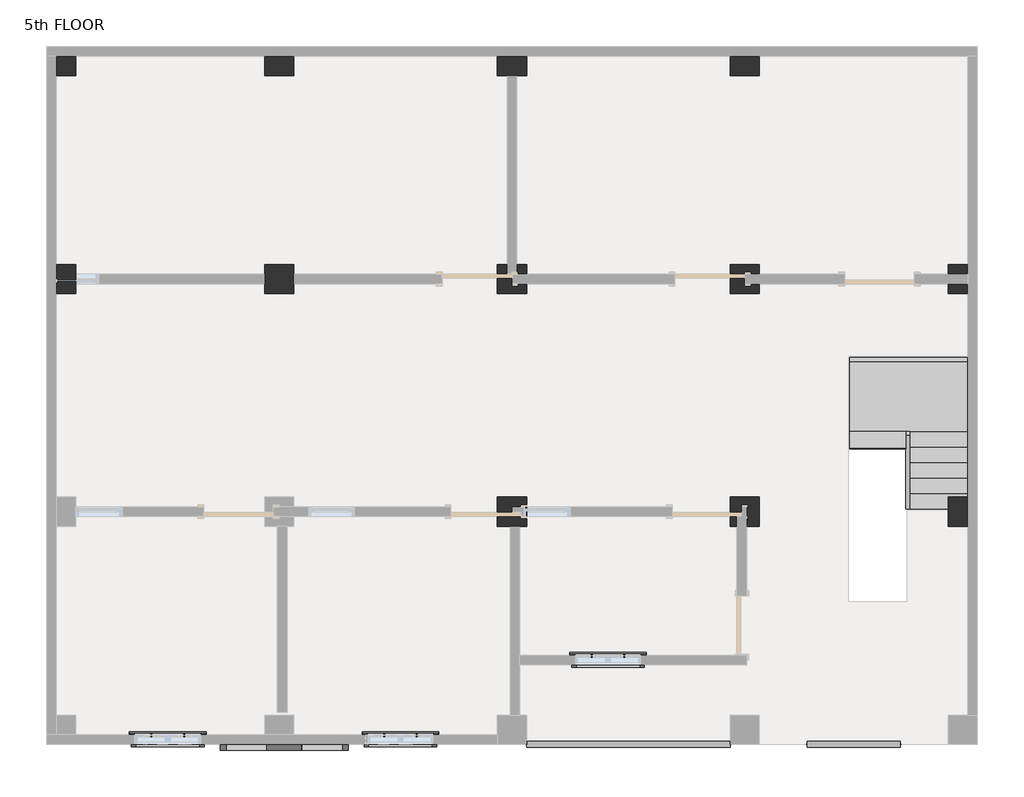
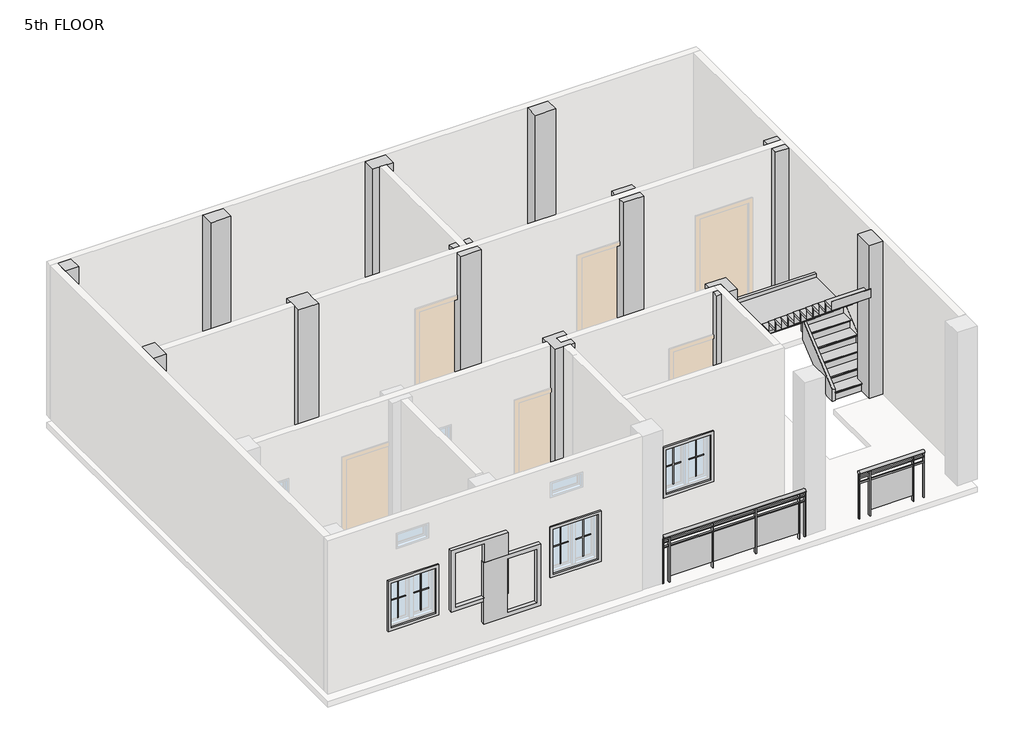
# One storey, part 2 of 2: 12 columns, 12 proxies, 4 members, 2 railings, 1 damper, 1 stair flight.
"""IFC4 building model written with IfcOpenShell, lengths in millimetres."""

from ifc_helpers import new_model, si_unit, point, frame, origin, place, context, project, spatial, polyline, ellipse_curve, trimmed, outline, extrude, faceted_brep, transform, mapped, element, save
from ifc_brep_helpers import plane_surface, extruded_surface, advanced_brep
from components import muntin_pattern_2x2_muntin_pattern_2x2_b3fe6957, muntin_pattern_2x2_muntin_pattern_2x2_3e0ecaf2, trim_window_exterior_flat_with_sill_41619996, trim_window_interior_flat_picture_frame_51c85655, duct_accessories_8_duct_accessories_1_4ac22e68, stair_flight_9ad1fb7f

model = new_model("IFC4")

# Units and contexts
model_context = context("Model", 3, world=origin())
ifc_project = project(units=[si_unit("LENGTHUNIT", "METRE", prefix="MILLI")], contexts=[model_context])

# Site, building, storey
site = spatial("IfcSite", under=ifc_project)
building = spatial("IfcBuilding", under=site)
storey = spatial("IfcBuildingStorey", under=building, Name="5th FLOOR", Elevation=15087.6)

# Proxies
placement = place(None, origin())
muntin_pattern_2x2_muntin_pattern_2x2_shape = muntin_pattern_2x2_muntin_pattern_2x2_b3fe6957(model_context)
element("IfcBuildingElementProxy", 1, Name="Muntin Pattern_2x2 : Muntin Pattern_2x2", ObjectType="Muntin Pattern_2x2 : Muntin Pattern_2x2", at=placement, inside=storey, context=model_context, shape_type="MappedRepresentation", body=[
    mapped(muntin_pattern_2x2_muntin_pattern_2x2_shape, transform((-14441.409625, -253.8184478, 16071.85), x_axis=(1.0, 0.0, 0.0), y_axis=(0.0, 1.0, 0.0), z_axis=(0.0, 0.0, 1.0))),
])
element("IfcBuildingElementProxy", 2, Name="Muntin Pattern_2x2 : Muntin Pattern_2x2", ObjectType="Muntin Pattern_2x2 : Muntin Pattern_2x2", at=placement, inside=storey, context=model_context, shape_type="MappedRepresentation", body=[
    mapped(muntin_pattern_2x2_muntin_pattern_2x2_shape, transform((-11393.409625, -253.8184478, 16071.85), x_axis=(1.0, 0.0, 0.0), y_axis=(0.0, 1.0, 0.0), z_axis=(0.0, 0.0, 1.0))),
])
element("IfcBuildingElementProxy", 3, Name="Muntin Pattern_2x2 : Muntin Pattern_2x2", ObjectType="Muntin Pattern_2x2 : Muntin Pattern_2x2", at=placement, inside=storey, context=model_context, shape_type="MappedRepresentation", body=[
    mapped(muntin_pattern_2x2_muntin_pattern_2x2_shape, transform((-8675.609625, 787.5815522, 16071.85), x_axis=(1.0, 0.0, 0.0), y_axis=(0.0, 1.0, 0.0), z_axis=(0.0, 0.0, 1.0))),
])
muntin_pattern_2x2_muntin_pattern_2x2_2_shape = muntin_pattern_2x2_muntin_pattern_2x2_3e0ecaf2(model_context)
element("IfcBuildingElementProxy", 4, Name="Muntin Pattern_2x2 : Muntin Pattern_2x2", ObjectType="Muntin Pattern_2x2 : Muntin Pattern_2x2", at=placement, inside=storey, context=model_context, shape_type="MappedRepresentation", body=[
    mapped(muntin_pattern_2x2_muntin_pattern_2x2_2_shape, transform((-14012.784625, -253.8184478, 16071.85), x_axis=(-1.0, 0.0, 0.0), y_axis=(0.0, -1.0, 0.0), z_axis=(0.0, 0.0, 1.0))),
])
element("IfcBuildingElementProxy", 5, Name="Muntin Pattern_2x2 : Muntin Pattern_2x2", ObjectType="Muntin Pattern_2x2 : Muntin Pattern_2x2", at=placement, inside=storey, context=model_context, shape_type="MappedRepresentation", body=[
    mapped(muntin_pattern_2x2_muntin_pattern_2x2_2_shape, transform((-10964.784625, -253.8184478, 16071.85), x_axis=(-1.0, 0.0, 0.0), y_axis=(0.0, -1.0, 0.0), z_axis=(0.0, 0.0, 1.0))),
])
element("IfcBuildingElementProxy", 6, Name="Muntin Pattern_2x2 : Muntin Pattern_2x2", ObjectType="Muntin Pattern_2x2 : Muntin Pattern_2x2", at=placement, inside=storey, context=model_context, shape_type="MappedRepresentation", body=[
    mapped(muntin_pattern_2x2_muntin_pattern_2x2_2_shape, transform((-8246.984625, 787.5815522, 16071.85), x_axis=(-1.0, 0.0, 0.0), y_axis=(0.0, -1.0, 0.0), z_axis=(0.0, 0.0, 1.0))),
])
trim_window_exterior_flat_with_sill_shape = trim_window_exterior_flat_with_sill_41619996(model_context)
element("IfcBuildingElementProxy", 7, Name="Trim-Window-Exterior-Flat : with Sill", ObjectType="Trim-Window-Exterior-Flat : with Sill", at=placement, inside=storey, context=model_context, shape_type="MappedRepresentation", body=[
    mapped(trim_window_exterior_flat_with_sill_shape, transform((-14227.097125, -244.2934478, 16916.4), x_axis=(-1.0, 0.0, 0.0), y_axis=(0.0, 0.0, 1.0), z_axis=(0.0, 1.0, 0.0))),
])
element("IfcBuildingElementProxy", 8, Name="Trim-Window-Exterior-Flat : with Sill", ObjectType="Trim-Window-Exterior-Flat : with Sill", at=placement, inside=storey, context=model_context, shape_type="MappedRepresentation", body=[
    mapped(trim_window_exterior_flat_with_sill_shape, transform((-11179.097125, -244.2934478, 16916.4), x_axis=(-1.0, 0.0, 0.0), y_axis=(0.0, 0.0, 1.0), z_axis=(0.0, 1.0, 0.0))),
])
element("IfcBuildingElementProxy", 9, Name="Trim-Window-Exterior-Flat : with Sill", ObjectType="Trim-Window-Exterior-Flat : with Sill", at=placement, inside=storey, context=model_context, shape_type="MappedRepresentation", body=[
    mapped(trim_window_exterior_flat_with_sill_shape, transform((-8461.297125, 797.1065522, 16916.4), x_axis=(-1.0, 0.0, 0.0), y_axis=(0.0, 0.0, 1.0), z_axis=(0.0, 1.0, 0.0))),
])
trim_window_interior_flat_picture_frame_shape = trim_window_interior_flat_picture_frame_51c85655(model_context)
element("IfcBuildingElementProxy", 10, Name="Trim-Window-Interior-Flat : Picture Frame", ObjectType="Trim-Window-Interior-Flat : Picture Frame", at=placement, inside=storey, context=model_context, shape_type="MappedRepresentation", body=[
    mapped(trim_window_interior_flat_picture_frame_shape, transform((-14227.097125, -371.2934478, 16916.4), x_axis=(1.0, 0.0, 0.0), y_axis=(0.0, 0.0, 1.0), z_axis=(0.0, -1.0, 0.0))),
])
element("IfcBuildingElementProxy", 11, Name="Trim-Window-Interior-Flat : Picture Frame", ObjectType="Trim-Window-Interior-Flat : Picture Frame", at=placement, inside=storey, context=model_context, shape_type="MappedRepresentation", body=[
    mapped(trim_window_interior_flat_picture_frame_shape, transform((-11179.097125, -371.2934478, 16916.4), x_axis=(1.0, 0.0, 0.0), y_axis=(0.0, 0.0, 1.0), z_axis=(0.0, -1.0, 0.0))),
])
element("IfcBuildingElementProxy", 12, Name="Trim-Window-Interior-Flat : Picture Frame", ObjectType="Trim-Window-Interior-Flat : Picture Frame", at=placement, inside=storey, context=model_context, shape_type="MappedRepresentation", body=[
    mapped(trim_window_interior_flat_picture_frame_shape, transform((-8461.297125, 670.1065522, 16916.4), x_axis=(1.0, 0.0, 0.0), y_axis=(0.0, 0.0, 1.0), z_axis=(0.0, -1.0, 0.0))),
])

# Columns
element("IfcColumn", 13, ObjectType="column family : column family", at=placement, inside=storey, context=model_context, shape_type="SweptSolid", body=[
    extrude(outline(polyline([(-15433.597125, 8645.7065522), (-15433.597125, 8391.7065522), (-15687.597125, 8391.7065522), (-15687.597125, 8645.7065522), (-15433.597125, 8645.7065522)])), frame((0.0, 0.0, 15092.6), z_axis=(0.0, 0.0, 1.0), x_axis=(1.0, 0.0, 0.0)), (0.0, 0.0, 1.0), 3038.0),
])
element("IfcColumn", 14, ObjectType="column family : column family", at=placement, inside=storey, context=model_context, shape_type="SweptSolid", body=[
    extrude(outline(polyline([(-12576.097125, 5915.2065522), (-12576.097125, 5534.2065522), (-12957.097125, 5534.2065522), (-12957.097125, 5915.2065522), (-12576.097125, 5915.2065522)])), frame((0.0, 0.0, 15092.6), z_axis=(0.0, 0.0, 1.0), x_axis=(1.0, 0.0, 0.0)), (0.0, 0.0, 1.0), 3038.0),
])
element("IfcColumn", 15, ObjectType="column family : column family", at=placement, inside=storey, context=model_context, shape_type="Brep", body=[
    faceted_brep([(-9655.097125, 5915.2065522, 15092.6), (-9528.097125, 5915.2065522, 15092.6), (-9528.097125, 5788.2065522, 15092.6), (-9655.097125, 5788.2065522, 15092.6), (-9528.097125, 5915.2065522, 18130.6), (-9655.097125, 5915.2065522, 18130.6), (-9655.097125, 5788.2065522, 18130.6), (-9528.097125, 5788.2065522, 18130.6)], [[[0, 1, 2, 3]], [[4, 5, 6, 7]], [[0, 3, 6, 5]], [[4, 1, 0, 5]], [[3, 2, 7, 6]], [[1, 4, 7, 2]]]),
    faceted_brep([(-9528.097125, 5534.2065522, 18130.6), (-9528.097125, 5534.2065522, 15092.6), (-9528.097125, 5661.2065522, 15092.6), (-9528.097125, 5661.2065522, 18130.6), (-9909.097125, 5534.2065522, 15092.6), (-9909.097125, 5534.2065522, 18130.6), (-9909.097125, 5915.2065522, 15092.6), (-9909.097125, 5661.2065522, 18130.6), (-9909.097125, 5661.2065522, 17221.2), (-9909.097125, 5788.2065522, 17221.2), (-9909.097125, 5788.2065522, 18130.6), (-9909.097125, 5915.2065522, 18130.6), (-9782.097125, 5915.2065522, 18130.6), (-9782.097125, 5915.2065522, 15092.6), (-9782.097125, 5788.2065522, 15092.6), (-9782.097125, 5788.2065522, 18130.6), (-9782.097125, 5788.2065522, 17221.2), (-9718.597125, 5788.2065522, 15092.6), (-9718.597125, 5788.2065522, 17221.2), (-9718.597125, 5661.2065522, 15092.6), (-9718.597125, 5661.2065522, 17221.2)], [[[0, 1, 2, 3]], [[4, 1, 0, 5]], [[6, 4, 5, 7, 8, 9, 10, 11]], [[6, 11, 12, 13]], [[14, 13, 12, 15, 16]], [[17, 14, 16, 18]], [[19, 20, 8, 7, 3, 2]], [[1, 4, 6, 13, 14, 17, 19, 2]], [[5, 0, 3, 7]], [[12, 11, 10, 15]], [[9, 16, 15, 10]], [[18, 20, 19, 17]], [[20, 18, 16, 9, 8]]]),
])
element("IfcColumn", 16, ObjectType="column family : column family", at=placement, inside=storey, context=model_context, shape_type="Brep", body=[
    faceted_brep([(-6480.097125, 5534.2065522, 15092.6), (-6861.097125, 5534.2065522, 15092.6), (-6861.097125, 5915.2065522, 15092.6), (-6480.097125, 5915.2065522, 15092.6), (-6480.097125, 5788.2065522, 15092.6), (-6670.597125, 5788.2065522, 15092.6), (-6670.597125, 5661.2065522, 15092.6), (-6480.097125, 5661.2065522, 15092.6), (-6480.097125, 5534.2065522, 18130.6), (-6480.097125, 5661.2065522, 18130.6), (-6861.097125, 5534.2065522, 18130.6), (-6861.097125, 5661.2065522, 18130.6), (-6861.097125, 5661.2065522, 17221.2), (-6861.097125, 5788.2065522, 17221.2), (-6861.097125, 5788.2065522, 18130.6), (-6861.097125, 5915.2065522, 18130.6), (-6480.097125, 5915.2065522, 18130.6), (-6670.597125, 5661.2065522, 17221.2), (-6670.597125, 5788.2065522, 17221.2), (-6480.097125, 5788.2065522, 18130.6)], [[[0, 1, 2, 3, 4, 5, 6, 7]], [[8, 0, 7, 9]], [[1, 0, 8, 10]], [[2, 1, 10, 11, 12, 13, 14, 15]], [[3, 2, 15, 16]], [[10, 8, 9, 11]], [[6, 17, 12, 11, 9, 7]], [[13, 18, 5, 4, 19, 14]], [[3, 16, 19, 4]], [[16, 15, 14, 19]], [[18, 17, 6, 5]], [[17, 18, 13, 12]]]),
])
element("IfcColumn", 17, ObjectType="column family : column family", at=placement, inside=storey, context=model_context, shape_type="Brep", body=[
    faceted_brep([(-6480.097125, 2867.2065522, 15092.6), (-6480.097125, 2486.2065522, 15092.6), (-6645.197125, 2486.2065522, 15092.6), (-6645.197125, 2740.2065522, 15092.6), (-6708.697125, 2740.2065522, 15092.6), (-6708.697125, 2613.2065522, 15092.6), (-6772.197125, 2613.2065522, 15092.6), (-6772.197125, 2486.2065522, 15092.6), (-6861.097125, 2486.2065522, 15092.6), (-6861.097125, 2867.2065522, 15092.6), (-6480.097125, 2867.2065522, 18130.6), (-6480.097125, 2486.2065522, 18130.6), (-6861.097125, 2486.2065522, 18130.6), (-6772.197125, 2486.2065522, 18130.6), (-6861.097125, 2613.2065522, 18130.6), (-6861.097125, 2613.2065522, 17221.2), (-6861.097125, 2740.2065522, 17221.2), (-6861.097125, 2740.2065522, 18130.6), (-6861.097125, 2867.2065522, 18130.6), (-6772.197125, 2740.2065522, 18130.6), (-6645.197125, 2740.2065522, 18130.6), (-6645.197125, 2486.2065522, 18130.6), (-6772.197125, 2613.2065522, 18130.6), (-6772.197125, 2613.2065522, 17221.2), (-6772.197125, 2740.2065522, 17221.2), (-6708.697125, 2613.2065522, 17221.2), (-6708.697125, 2740.2065522, 17221.2)], [[[0, 1, 2, 3, 4, 5, 6, 7, 8, 9]], [[1, 0, 10, 11]], [[12, 8, 7, 13]], [[9, 8, 12, 14, 15, 16, 17, 18]], [[0, 9, 18, 10]], [[11, 10, 18, 17, 19, 20, 21]], [[15, 14, 22, 23]], [[17, 16, 24, 19]], [[20, 3, 2, 21]], [[6, 23, 22, 13, 7]], [[14, 12, 13, 22]], [[1, 11, 21, 2]], [[15, 23, 24, 16]], [[25, 23, 6, 5]], [[23, 25, 26, 24]], [[26, 25, 5, 4]], [[24, 26, 4, 3, 20, 19]]]),
])
element("IfcColumn", 18, ObjectType="column family : column family", at=placement, inside=storey, context=model_context, shape_type="Brep", body=[
    faceted_brep([(-9528.097125, 2486.2065522, 15092.6), (-9909.097125, 2486.2065522, 15092.6), (-9909.097125, 2867.2065522, 15092.6), (-9528.097125, 2867.2065522, 15092.6), (-9528.097125, 2740.2065522, 15092.6), (-9566.197125, 2740.2065522, 15092.6), (-9718.597125, 2740.2065522, 15092.6), (-9718.597125, 2613.2065522, 15092.6), (-9566.197125, 2613.2065522, 15092.6), (-9528.097125, 2613.2065522, 15092.6), (-9528.097125, 2486.2065522, 18130.6), (-9528.097125, 2613.2065522, 15392.4), (-9528.097125, 2740.2065522, 15392.4), (-9528.097125, 2867.2065522, 18130.6), (-9528.097125, 2740.2065522, 18130.6), (-9528.097125, 2740.2065522, 17221.2), (-9528.097125, 2613.2065522, 17221.2), (-9528.097125, 2613.2065522, 18130.6), (-9909.097125, 2486.2065522, 18130.6), (-9909.097125, 2867.2065522, 18130.6), (-9566.197125, 2613.2065522, 18130.6), (-9718.597125, 2613.2065522, 18130.6), (-9718.597125, 2740.2065522, 18130.6), (-9566.197125, 2740.2065522, 18130.6), (-9566.197125, 2613.2065522, 17221.2), (-9566.197125, 2613.2065522, 15392.4), (-9566.197125, 2740.2065522, 15392.4), (-9566.197125, 2740.2065522, 17221.2)], [[[0, 1, 2, 3, 4, 5, 6, 7, 8, 9]], [[10, 0, 9, 11, 12, 4, 3, 13, 14, 15, 16, 17]], [[1, 0, 10, 18]], [[2, 1, 18, 19]], [[3, 2, 19, 13]], [[18, 10, 17, 20, 21, 22, 23, 14, 13, 19]], [[11, 9, 8, 7, 21, 20, 17, 16, 24, 25]], [[4, 12, 26, 27, 15, 14, 23, 22, 6, 5]], [[21, 7, 6, 22]], [[25, 24, 27, 26]], [[25, 26, 12, 11]], [[27, 24, 16, 15]]]),
])
element("IfcColumn", 19, ObjectType="column family : column family", at=placement, inside=storey, context=model_context, shape_type="SweptSolid", body=[
    extrude(outline(polyline([(-12576.097125, 8391.7065522), (-12957.097125, 8391.7065522), (-12957.097125, 8645.7065522), (-12576.097125, 8645.7065522), (-12576.097125, 8391.7065522)])), frame((0.0, 0.0, 15092.6), z_axis=(0.0, 0.0, 1.0), x_axis=(1.0, 0.0, 0.0)), (0.0, 0.0, 1.0), 3038.0),
])
element("IfcColumn", 20, ObjectType="column family : column family", at=placement, inside=storey, context=model_context, shape_type="SweptSolid", body=[
    extrude(outline(polyline([(-9528.097125, 8391.7065522), (-9909.097125, 8391.7065522), (-9909.097125, 8645.7065522), (-9528.097125, 8645.7065522), (-9528.097125, 8391.7065522)])), frame((0.0, 0.0, 15092.6), z_axis=(0.0, 0.0, 1.0), x_axis=(1.0, 0.0, 0.0)), (0.0, 0.0, 1.0), 3038.0),
])
element("IfcColumn", 21, ObjectType="column family : column family", at=placement, inside=storey, context=model_context, shape_type="SweptSolid", body=[
    extrude(outline(polyline([(-6480.097125, 8391.7065522), (-6861.097125, 8391.7065522), (-6861.097125, 8645.7065522), (-6480.097125, 8645.7065522), (-6480.097125, 8391.7065522)])), frame((0.0, 0.0, 15092.6), z_axis=(0.0, 0.0, 1.0), x_axis=(1.0, 0.0, 0.0)), (0.0, 0.0, 1.0), 3038.0),
])
element("IfcColumn", 22, ObjectType="column family : column family", at=placement, inside=storey, context=model_context, shape_type="SweptSolid", body=[
    extrude(outline(polyline([(-4003.597125, 5915.2065522), (-3749.597125, 5915.2065522), (-3749.597125, 5788.2065522), (-4003.597125, 5788.2065522), (-4003.597125, 5915.2065522)])), frame((0.0, 0.0, 15092.6), z_axis=(0.0, 0.0, 1.0), x_axis=(1.0, 0.0, 0.0)), (0.0, 0.0, 1.0), 3038.0),
    extrude(outline(polyline([(-3749.597125, 5534.2065522), (-4003.597125, 5534.2065522), (-4003.597125, 5661.2065522), (-3749.597125, 5661.2065522), (-3749.597125, 5534.2065522)])), frame((0.0, 0.0, 15092.6), z_axis=(0.0, 0.0, 1.0), x_axis=(1.0, 0.0, 0.0)), (0.0, 0.0, 1.0), 3038.0),
])
element("IfcColumn", 23, ObjectType="column family : column family", at=placement, inside=storey, context=model_context, shape_type="SweptSolid", body=[
    extrude(outline(polyline([(-4003.597125, 2486.2065522), (-4003.597125, 2867.2065522), (-3749.597125, 2867.2065522), (-3749.597125, 2486.2065522), (-4003.597125, 2486.2065522)])), frame((0.0, 0.0, 15092.6), z_axis=(0.0, 0.0, 1.0), x_axis=(1.0, 0.0, 0.0)), (0.0, 0.0, 1.0), 3038.0),
])
element("IfcColumn", 24, ObjectType="column family : column family", at=placement, inside=storey, context=model_context, shape_type="SweptSolid", body=[
    extrude(outline(polyline([(-15433.597125, 5915.2065522), (-15433.597125, 5534.2065522), (-15687.597125, 5534.2065522), (-15687.597125, 5915.2065522), (-15433.597125, 5915.2065522)])), frame((0.0, 0.0, 15092.6), z_axis=(0.0, 0.0, 1.0), x_axis=(1.0, 0.0, 0.0)), (0.0, 0.0, 1.0), 3038.0),
])

# Damper
duct_accessories_8_duct_accessories_1_shape = duct_accessories_8_duct_accessories_1_4ac22e68(model_context)
element("IfcDamper", 25, ObjectType="Duct Accessories 8 : Duct Accessories 1", at=placement, inside=storey, context=model_context, shape_type="MappedRepresentation", body=[
    mapped(duct_accessories_8_duct_accessories_1_shape, transform((0.0, 0.0, 0.0), x_axis=(1.0, 0.0, 0.0), y_axis=(0.0, 1.0, 0.0), z_axis=(0.0, 0.0, 1.0))),
])

# Members
element("IfcMember", 26, ObjectType="Stringer - 2\" Width", at=placement, inside=storey, context=model_context, shape_type="SweptSolid", body=[
    extrude(outline(polyline([(2714.6319226, 15087.6), (2714.6319226, 15324.4438745), (3679.8319226, 16128.7772078), (3679.8319226, 15732.0165243), (2906.5320935, 15087.6), (2714.6319226, 15087.6)])), frame((-4563.0136682, 0.0, 0.0), z_axis=(1.0, 0.0, 0.0), x_axis=(0.0, 1.0, 0.0)), (0.0, 0.0, 1.0), 50.8),
])
element("IfcMember", 27, ObjectType="Stringer - 2\" Width", at=placement, inside=storey, context=model_context, shape_type="SweptSolid", body=[
    extrude(outline(polyline([(-4512.2136682, 3730.6319226), (-4512.2136682, 3679.8319226), (-4563.0136682, 3679.8319226), (-4563.0136682, 3730.6319226), (-4512.2136682, 3730.6319226)])), frame((0.0, 0.0, 15875.0), z_axis=(0.0, 0.0, 1.0), x_axis=(1.0, 0.0, 0.0)), (0.0, 0.0, 1.0), 304.8),
])
element("IfcMember", 28, ObjectType="Stringer - 2\" Width", at=placement, inside=storey, context=model_context, shape_type="SweptSolid", body=[
    extrude(outline(polyline([(2714.6319226, 15087.6), (2714.6319226, 15324.4438745), (3741.0592732, 16179.8), (4217.1720935, 16179.8), (2906.5320935, 15087.6), (2714.6319226, 15087.6)])), frame((-3749.597125, 0.0, 0.0), z_axis=(1.0, 0.0, 0.0), x_axis=(0.0, 1.0, 0.0)), (0.0, 0.0, 1.0), 50.8),
])
element("IfcMember", 29, ObjectType="Stringer - 2\" Width", at=placement, inside=storey, context=model_context, shape_type="SweptSolid", body=[
    extrude(outline(polyline([(-3698.797125, 4695.8319226), (-3698.797125, 4645.0319226), (-5295.0246464, 4645.0319226), (-5295.0246464, 4695.8319226), (-3698.797125, 4695.8319226)])), frame((0.0, 0.0, 15875.0), z_axis=(0.0, 0.0, 1.0), x_axis=(1.0, 0.0, 0.0)), (0.0, 0.0, 1.0), 304.8),
])

# Railings
element("IfcRailing", 30, ObjectType="Glass Panel - Bottom Fill", at=placement, inside=storey, context=model_context, shape_type="SolidModel", body=[
    advanced_brep(
    [(-9528.097125, -333.1934478, 16002.0), (-9528.097125, -409.3934478, 16002.0), (-6861.097125, -333.1934478, 16002.0), (-6861.097125, -409.3934478, 16002.0)],
    [
        (0, 1, ellipse_curve(frame((-9528.097125, -371.2934478, 16002.0), z_axis=(-1.0, 0.0, 0.0), x_axis=(0.0, -1.0, 0.0)), 38.1, 28.575)),
        (1, 0, ellipse_curve(frame((-9528.097125, -371.2934478, 16002.0), z_axis=(-1.0, 0.0, 0.0), x_axis=(0.0, -1.0, 0.0)), 38.1, 28.575)),
        (2, 3, ellipse_curve(frame((-6861.097125, -371.2934478, 16002.0), z_axis=(1.0, 0.0, 0.0), x_axis=(0.0, -1.0, 0.0)), 38.1, 28.575)),
        (3, 2, ellipse_curve(frame((-6861.097125, -371.2934478, 16002.0), z_axis=(1.0, 0.0, 0.0), x_axis=(0.0, -1.0, 0.0)), 38.1, 28.575)),
        (0, 2),
        (3, 1),
    ],
    [
        plane_surface(frame((-9528.097125, -371.2934478, 16002.0), z_axis=(-1.0, 0.0, 0.0), x_axis=(0.0, 1.0, 0.0))),
        plane_surface(frame((-6861.097125, -371.2934478, 16002.0), z_axis=(1.0, 0.0, 0.0), x_axis=(0.0, 1.0, 0.0))),
        extruded_surface(trimmed(ellipse_curve(frame((-6861.097125, -371.2934478, 16002.0), z_axis=(-1.0, 0.0, 0.0), x_axis=(0.0, -1.0, 0.0)), 38.1, 28.575), [point((-6861.097125, -333.1934478, 16002.0))], [point((-6861.097125, -409.3934478, 16002.0))], True, "CARTESIAN"), (-2667.0, 0.0, 0.0), 2667.0),
        extruded_surface(trimmed(ellipse_curve(frame((-6861.097125, -371.2934478, 16002.0), z_axis=(-1.0, 0.0, 0.0), x_axis=(0.0, -1.0, 0.0)), 38.1, 28.575), [point((-6861.097125, -409.3934478, 16002.0))], [point((-6861.097125, -333.1934478, 16002.0))], True, "CARTESIAN"), (-2667.0, 0.0, 0.0), 2667.0),
    ],
    [
        (0, [[1, 2]]),
        (1, [[3, 4]]),
        (2, [[-1, 5, -4, 6]]),
        (3, [[-2, -6, -3, -5]]),
    ],
),
    extrude(outline(polyline([(-9528.097125, -383.9934478), (-9528.097125, -358.5934478), (-6861.097125, -358.5934478), (-6861.097125, -383.9934478), (-9528.097125, -383.9934478)])), frame((0.0, 0.0, 15887.7), z_axis=(0.0, 0.0, 1.0), x_axis=(1.0, 0.0, 0.0)), (0.0, 0.0, 1.0), 25.4),
    extrude(outline(polyline([(-9528.097125, -383.9934478), (-9528.097125, -358.5934478), (-6861.097125, -358.5934478), (-6861.097125, -383.9934478), (-9528.097125, -383.9934478)])), frame((0.0, 0.0, 15786.1), z_axis=(0.0, 0.0, 1.0), x_axis=(1.0, 0.0, 0.0)), (0.0, 0.0, 1.0), 25.4),
    extrude(outline(polyline([(-6981.747125, -396.6934478), (-6981.747125, -345.8934478), (-6969.047125, -345.8934478), (-6969.047125, -396.6934478), (-6981.747125, -396.6934478)])), frame((0.0, 0.0, 15087.6), z_axis=(0.0, 0.0, 1.0), x_axis=(1.0, 0.0, 0.0)), (0.0, 0.0, 1.0), 885.6788223),
    extrude(outline(polyline([(-7788.197125, -364.7582908), (-6975.397125, -364.7582908), (-6975.397125, -371.1082908), (-7788.197125, -371.1082908), (-7788.197125, -364.7582908)])), frame((0.0, 0.0, 15189.2), z_axis=(0.0, 0.0, 1.0), x_axis=(1.0, 0.0, 0.0)), (0.0, 0.0, 1.0), 596.9),
    extrude(outline(polyline([(-7794.547125, -396.6934478), (-7794.547125, -345.8934478), (-7781.847125, -345.8934478), (-7781.847125, -396.6934478), (-7794.547125, -396.6934478)])), frame((0.0, 0.0, 15087.6), z_axis=(0.0, 0.0, 1.0), x_axis=(1.0, 0.0, 0.0)), (0.0, 0.0, 1.0), 885.6788223),
    extrude(outline(polyline([(-8600.997125, -364.7582908), (-7788.197125, -364.7582908), (-7788.197125, -371.1082908), (-8600.997125, -371.1082908), (-8600.997125, -364.7582908)])), frame((0.0, 0.0, 15189.2), z_axis=(0.0, 0.0, 1.0), x_axis=(1.0, 0.0, 0.0)), (0.0, 0.0, 1.0), 596.9),
    extrude(outline(polyline([(-8607.347125, -396.6934478), (-8607.347125, -345.8934478), (-8594.647125, -345.8934478), (-8594.647125, -396.6934478), (-8607.347125, -396.6934478)])), frame((0.0, 0.0, 15087.6), z_axis=(0.0, 0.0, 1.0), x_axis=(1.0, 0.0, 0.0)), (0.0, 0.0, 1.0), 885.6788223),
    extrude(outline(polyline([(-9413.797125, -364.7582908), (-8600.997125, -364.7582908), (-8600.997125, -371.1082908), (-9413.797125, -371.1082908), (-9413.797125, -364.7582908)])), frame((0.0, 0.0, 15189.2), z_axis=(0.0, 0.0, 1.0), x_axis=(1.0, 0.0, 0.0)), (0.0, 0.0, 1.0), 596.9),
    extrude(outline(polyline([(-9420.147125, -396.6934478), (-9420.147125, -345.8934478), (-9407.447125, -345.8934478), (-9407.447125, -396.6934478), (-9420.147125, -396.6934478)])), frame((0.0, 0.0, 15087.6), z_axis=(0.0, 0.0, 1.0), x_axis=(1.0, 0.0, 0.0)), (0.0, 0.0, 1.0), 885.6788223),
    extrude(outline(polyline([(-6873.797125, -380.8184478), (-6873.797125, -361.7684478), (-6854.747125, -361.7684478), (-6854.747125, -380.8184478), (-6873.797125, -380.8184478)])), frame((0.0, 0.0, 15087.6), z_axis=(0.0, 0.0, 1.0), x_axis=(1.0, 0.0, 0.0)), (0.0, 0.0, 1.0), 885.6788223),
    extrude(outline(polyline([(-9534.447125, -380.8184478), (-9534.447125, -361.7684478), (-9515.397125, -361.7684478), (-9515.397125, -380.8184478), (-9534.447125, -380.8184478)])), frame((0.0, 0.0, 15087.6), z_axis=(0.0, 0.0, 1.0), x_axis=(1.0, 0.0, 0.0)), (0.0, 0.0, 1.0), 885.6788223),
])
element("IfcRailing", 31, ObjectType="Glass Panel - Bottom Fill", at=placement, inside=storey, context=model_context, shape_type="SolidModel", body=[
    advanced_brep(
    [(-5851.447125, -333.1934478, 16002.0), (-5851.447125, -409.3934478, 16002.0), (-4632.247125, -333.1934478, 16002.0), (-4632.247125, -409.3934478, 16002.0)],
    [
        (0, 1, ellipse_curve(frame((-5851.447125, -371.2934478, 16002.0), z_axis=(-1.0, 0.0, 0.0), x_axis=(0.0, -1.0, 0.0)), 38.1, 28.575)),
        (1, 0, ellipse_curve(frame((-5851.447125, -371.2934478, 16002.0), z_axis=(-1.0, 0.0, 0.0), x_axis=(0.0, -1.0, 0.0)), 38.1, 28.575)),
        (2, 3, ellipse_curve(frame((-4632.247125, -371.2934478, 16002.0), z_axis=(1.0, 0.0, 0.0), x_axis=(0.0, -1.0, 0.0)), 38.1, 28.575)),
        (3, 2, ellipse_curve(frame((-4632.247125, -371.2934478, 16002.0), z_axis=(1.0, 0.0, 0.0), x_axis=(0.0, -1.0, 0.0)), 38.1, 28.575)),
        (0, 2),
        (3, 1),
    ],
    [
        plane_surface(frame((-5851.447125, -371.2934478, 16002.0), z_axis=(-1.0, 0.0, 0.0), x_axis=(0.0, 1.0, 0.0))),
        plane_surface(frame((-4632.247125, -371.2934478, 16002.0), z_axis=(1.0, 0.0, 0.0), x_axis=(0.0, 1.0, 0.0))),
        extruded_surface(trimmed(ellipse_curve(frame((-4632.247125, -371.2934478, 16002.0), z_axis=(-1.0, 0.0, 0.0), x_axis=(0.0, -1.0, 0.0)), 38.1, 28.575), [point((-4632.247125, -333.1934478, 16002.0))], [point((-4632.247125, -409.3934478, 16002.0))], True, "CARTESIAN"), (-1219.1999999999998, 0.0, 0.0), 1219.1999999999998),
        extruded_surface(trimmed(ellipse_curve(frame((-4632.247125, -371.2934478, 16002.0), z_axis=(-1.0, 0.0, 0.0), x_axis=(0.0, -1.0, 0.0)), 38.1, 28.575), [point((-4632.247125, -409.3934478, 16002.0))], [point((-4632.247125, -333.1934478, 16002.0))], True, "CARTESIAN"), (-1219.1999999999998, 0.0, 0.0), 1219.1999999999998),
    ],
    [
        (0, [[1, 2]]),
        (1, [[3, 4]]),
        (2, [[-1, 5, -4, 6]]),
        (3, [[-2, -6, -3, -5]]),
    ],
),
    extrude(outline(polyline([(-5851.447125, -383.9934478), (-5851.447125, -358.5934478), (-4632.247125, -358.5934478), (-4632.247125, -383.9934478), (-5851.447125, -383.9934478)])), frame((0.0, 0.0, 15887.7), z_axis=(0.0, 0.0, 1.0), x_axis=(1.0, 0.0, 0.0)), (0.0, 0.0, 1.0), 25.4),
    extrude(outline(polyline([(-5851.447125, -383.9934478), (-5851.447125, -358.5934478), (-4632.247125, -358.5934478), (-4632.247125, -383.9934478), (-5851.447125, -383.9934478)])), frame((0.0, 0.0, 15786.1), z_axis=(0.0, 0.0, 1.0), x_axis=(1.0, 0.0, 0.0)), (0.0, 0.0, 1.0), 25.4),
    extrude(outline(polyline([(-4841.797125, -396.6934478), (-4841.797125, -345.8934478), (-4829.097125, -345.8934478), (-4829.097125, -396.6934478), (-4841.797125, -396.6934478)])), frame((0.0, 0.0, 15087.6), z_axis=(0.0, 0.0, 1.0), x_axis=(1.0, 0.0, 0.0)), (0.0, 0.0, 1.0), 885.6788223),
    extrude(outline(polyline([(-5648.247125, -364.7582908), (-4835.447125, -364.7582908), (-4835.447125, -371.1082908), (-5648.247125, -371.1082908), (-5648.247125, -364.7582908)])), frame((0.0, 0.0, 15189.2), z_axis=(0.0, 0.0, 1.0), x_axis=(1.0, 0.0, 0.0)), (0.0, 0.0, 1.0), 596.9),
    extrude(outline(polyline([(-5654.597125, -396.6934478), (-5654.597125, -345.8934478), (-5641.897125, -345.8934478), (-5641.897125, -396.6934478), (-5654.597125, -396.6934478)])), frame((0.0, 0.0, 15087.6), z_axis=(0.0, 0.0, 1.0), x_axis=(1.0, 0.0, 0.0)), (0.0, 0.0, 1.0), 885.6788223),
    extrude(outline(polyline([(-4644.947125, -380.8184478), (-4644.947125, -361.7684478), (-4625.897125, -361.7684478), (-4625.897125, -380.8184478), (-4644.947125, -380.8184478)])), frame((0.0, 0.0, 15087.6), z_axis=(0.0, 0.0, 1.0), x_axis=(1.0, 0.0, 0.0)), (0.0, 0.0, 1.0), 885.6788223),
    extrude(outline(polyline([(-5857.797125, -380.8184478), (-5857.797125, -361.7684478), (-5838.747125, -361.7684478), (-5838.747125, -380.8184478), (-5857.797125, -380.8184478)])), frame((0.0, 0.0, 15087.6), z_axis=(0.0, 0.0, 1.0), x_axis=(1.0, 0.0, 0.0)), (0.0, 0.0, 1.0), 885.6788223),
])

# Stair flight
stair_flight_shape = stair_flight_9ad1fb7f(model_context)
element("IfcStairFlight", 32, ObjectType="2\" Tread 1\" Nosing 1/4\" Riser", at=placement, inside=storey, context=model_context, shape_type="MappedRepresentation", body=[
    mapped(stair_flight_shape, transform((0.0, 0.0, 0.0), x_axis=(1.0, 0.0, 0.0), y_axis=(0.0, 1.0, 0.0), z_axis=(0.0, 0.0, 1.0))),
])

save(model, "model.ifc")

# Revit data of these elements
# Type "Muntin Pattern_2x2 : Muntin Pattern_2x2"
#   Width [instance default] = 4' - 0"
#   Thickness = 0' - 0 1/2"
#   Height [instance default] = 4' - 0"
#   Distance = 0' - 0 3/4"
#   Interior Material [instance default] = none
#   Exterior Material [instance default] = none
#   Default Elevation = 0
# Type "Trim-Window-Exterior-Flat : with Sill"
#   Trim Width = 0' - 2 1/4"
#   Trim Thickness_Picture Frame = 0' - 1 1/4"
#   Trim Thickness_with Sill = 0' - 0 3/4"
#   Sill Thickness = 0' - 1 1/4"
#   Opening Width [instance default] = 2' - 0"
#   Opening Height [instance default] = 3' - 0"
#   Default Elevation = 4' - 0"
#   Sill = yes
#   Picture Frame = no
#   Trim Material [instance default] = none
# Type "Trim-Window-Interior-Flat : Picture Frame"
#   Trim Thickness_Picture Frame = 0' - 1 1/4"
#   Trim Width = 0' - 2 1/4"
#   Trim Thickness_with Sill = 0' - 0 3/4"
#   Sill Thickness = 0' - 1 1/4"
#   Opening Width [instance default] = 2' - 0"
#   Opening Height [instance default] = 3' - 0"
#   Default Elevation = 4' - 0"
#   Sill = no
#   Picture Frame = yes
#   Trim Material [instance default] = none
# Type "column family : column family"
#   w2 [instance default] = 0' - 9.88189"
#   w1 [instance default] = 0' - 9.01575"
#   Depth = 1' - 11.62205"
#   Width = 1' - 11.62205"
# Type "Glass Panel - Bottom Fill"
#   Assembly Code = "C2010400"
#   built-in parameter 1008612 = 0.0416667 (stored number, unit not read)
#   built-in parameter 1008611 = 0.0416667 (stored number, unit not read)
#   built-in parameter 1008609 = 0.333333 (stored number, unit not read)
#   built-in parameter 1008604 = 0.166667 (stored number, unit not read)
#   built-in parameter 1008603 = 0.166667 (stored number, unit not read)
#   Railing Height = 3' - 0"
#   built-in parameter 1008630 = 2
#   built-in parameter 1008610 = 2
#   built-in parameter 1008618 = Baluster - Square : 3/4"
# Elements 1, 2, 3, 4, 5, 6 (IfcBuildingElementProxy, "Muntin Pattern_2x2 : Muntin Pattern_2x2")
#   Width = 0' - 11 5/8"
#   Height = 2' - 6 1/2"
#   Interior Material = Wood - Stained
#   Exterior Material = Clad - White
#   Phase Created = New Construction
#   Materials on its faces: "Clad - White", "Wood - Stained"
# Elements 7, 8, 9 (IfcBuildingElementProxy, "Trim-Window-Exterior-Flat : with Sill")
#   Opening Width = 2' - 10"
#   Opening Height = 3' - 0"
#   Trim Material = Clad - White
#   Phase Created = New Construction
#   Materials on its faces: "Clad - White"
# Elements 10, 11, 12 (IfcBuildingElementProxy, "Trim-Window-Interior-Flat : Picture Frame")
#   Opening Width = 2' - 10"
#   Opening Height = 3' - 0"
#   Trim Material = Wood - Stained
#   Phase Created = New Construction
#   Materials on its faces: "Wood - Stained"
# Elements 13, 14, 15, 19, 20, 21 (IfcColumn, "column family : column family")
#   w2 = 1' - 3"
#   w1 = 1' - 3"
#   Phase Created = New Construction
#   Materials on its faces: "Default Wall"
# Elements 16, 22, 23 (IfcColumn, "column family : column family")
#   w2 = 1' - 3"
#   w1 = 1' - 3"
#   Phase Created = New Construction
#   Materials on its faces: "grey", "Default Wall"
# Elements 17, 18 (IfcColumn, "column family : column family")
#   w2 = 1' - 3"
#   w1 = 1' - 3"
#   Phase Created = New Construction
#   Materials on its faces: "Default Wall", "inside wall"
# Element 24 (IfcColumn, "column family : column family")
#   w2 = 1' - 3"
#   w1 = 1' - 3"
#   Phase Created = New Construction
#   Materials on its faces: "inside wall", "Default Wall"
# Element 25 (IfcDamper, "Duct Accessories 8 : Duct Accessories 1")
#   Mark = "8"
#   Phase Created = New Construction
#   Materials on its faces: "border"
# Elements 26, 27, 28, 29 (IfcMember, "Stringer - 2\" Width")
#   Phase Created = New Construction
# Elements 30, 31 (IfcRailing, "Glass Panel - Bottom Fill")
#   Phase Created = New Construction
#   Materials on its faces: "Glass"
# Element 32 (IfcStairFlight, "2\" Tread 1\" Nosing 1/4\" Riser")
#   Phase Created = New Construction
# Materials
#   "Clad - White": class "Wood", colour RGB 242 242 238, transparency 0, Cost = 0
#   "Wood - Stained": class "Wood", colour RGB 224 178 126, transparency 0, Cost = 0
#   "Default Wall": colour RGB 128 128 128, transparency 0, Cost = 0
#   "grey": class "Generic", colour RGB 80 80 80, transparency 0, Cost = 0
#   "inside wall": class "Generic", colour RGB 199 224 95, transparency 0, Cost = 0
#   "border": class "Generic", colour RGB 144 144 144, transparency 0, Cost = 0
#   "Glass": class "Glass", colour RGB 0 128 192, transparency 0.75, Description = "Soda Lime Glass", Cost = 0
